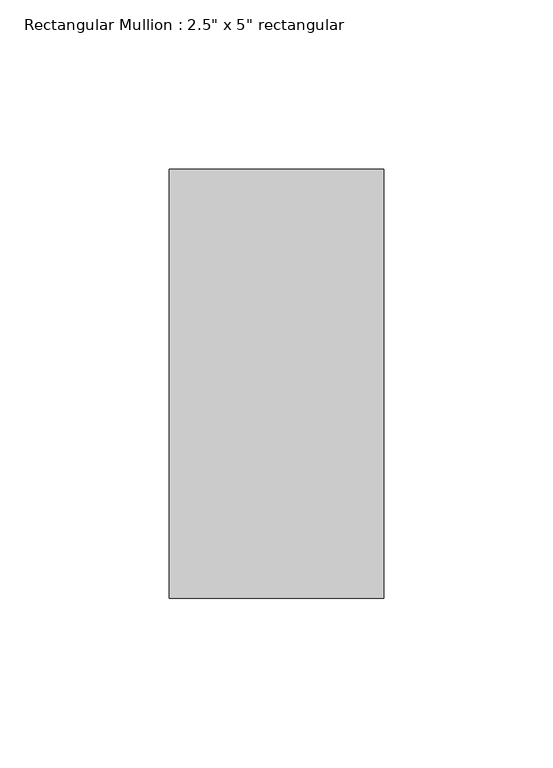
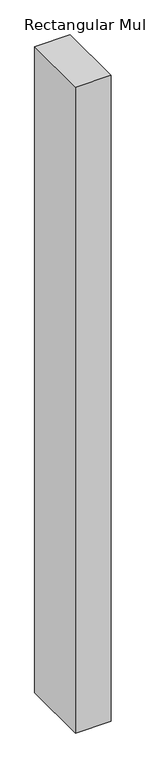
"""IFC4 building model written with IfcOpenShell, lengths in millimetres: member geometry."""

from ifc_helpers import new_model, si_unit, frame, origin, place, context, project, spatial, polyline, outline, extrude, source, transform, mapped, element, save


def member_86232e3a(model_context):
    return source(origin(), model_context, "Body", "SweptSolid", [
        extrude(outline(polyline([(0.0, 63.5), (0.0, -63.5), (-63.5, -63.5), (-63.5, 63.5), (0.0, 63.5)])), frame((0.0, 0.0, -1225.5500001), z_axis=(0.0, 0.0, 1.0), x_axis=(1.0, 0.0, 0.0)), (0.0, 0.0, 1.0), 1225.5500001),
    ])


if __name__ == "__main__":
    model = new_model("IFC4")
    model_context = context("Model", 3, world=origin())
    ifc_project = project(units=[si_unit("LENGTHUNIT", "METRE", prefix="MILLI")], contexts=[model_context])
    site = spatial("IfcSite", under=ifc_project)
    building = spatial("IfcBuilding", under=site)
    placement = place(None, origin())
    member_shape = member_86232e3a(model_context)
    element("IfcMember", 1, ObjectType="Rectangular Mullion : 2.5\" x 5\" rectangular", at=placement, inside=building, context=model_context, shape_type="MappedRepresentation", body=[
        mapped(member_shape, transform((0.0, 0.0, 0.0), x_axis=(1.0, 0.0, 0.0), y_axis=(0.0, 1.0, 0.0), z_axis=(0.0, 0.0, 1.0))),
    ])
    save(model, "model.ifc")

# Revit data of these elements
# Type "Rectangular Mullion : 2.5\" x 5\" rectangular"
#   built-in parameter 1007304 = 0.416667 (stored number, unit not read)
#   built-in parameter 1007301 = 0.104167 (stored number, unit not read)
#   built-in parameter 1007300 = 0.104167 (stored number, unit not read)
# Element 1 (IfcMember, "Rectangular Mullion : 2.5\" x 5\" rectangular")
#   Materials on its faces: "Aluminum"
# Materials
#   "Aluminum": class "Metal", colour RGB 247 247 247, transparency 0, Description = "Aluminum 6061", Cost = 0
